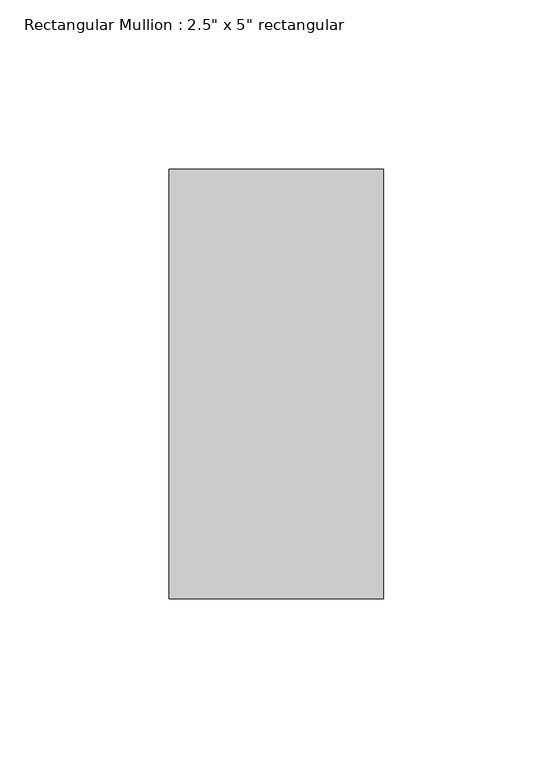
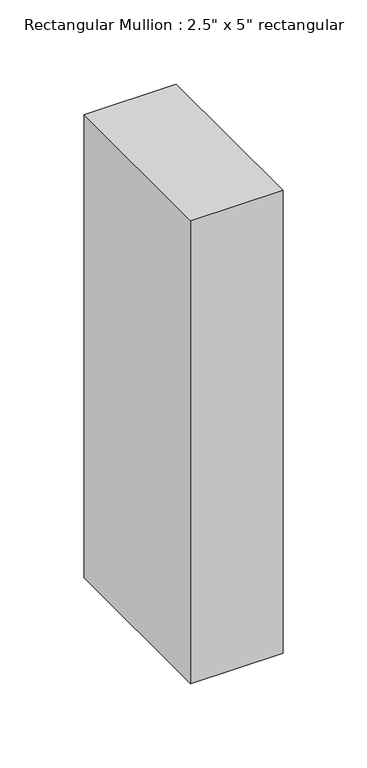
"""IFC4 building model written with IfcOpenShell, lengths in millimetres: member geometry."""

from ifc_helpers import new_model, si_unit, frame, origin, place, context, project, spatial, polyline, outline, extrude, source, transform, mapped, element, save


def member_02b8d6b6(model_context):
    return source(origin(), model_context, "Body", "SweptSolid", [
        extrude(outline(polyline([(0.0, 63.5), (0.0, -63.5), (-63.5, -63.5), (-63.5, 63.5), (0.0, 63.5)])), frame((0.0, 0.0, -336.55), z_axis=(0.0, 0.0, 1.0), x_axis=(1.0, 0.0, 0.0)), (0.0, 0.0, 1.0), 336.55),
    ])


if __name__ == "__main__":
    model = new_model("IFC4")
    model_context = context("Model", 3, world=origin())
    ifc_project = project(units=[si_unit("LENGTHUNIT", "METRE", prefix="MILLI")], contexts=[model_context])
    site = spatial("IfcSite", under=ifc_project)
    building = spatial("IfcBuilding", under=site)
    placement = place(None, origin())
    member_shape = member_02b8d6b6(model_context)
    element("IfcMember", 1, ObjectType="Rectangular Mullion : 2.5\" x 5\" rectangular", at=placement, inside=building, context=model_context, shape_type="MappedRepresentation", body=[
        mapped(member_shape, transform((0.0, 0.0, 0.0), x_axis=(1.0, 0.0, 0.0), y_axis=(0.0, 1.0, 0.0), z_axis=(0.0, 0.0, 1.0))),
    ])
    save(model, "model.ifc")

# Revit data of these elements
# Type "Rectangular Mullion : 2.5\" x 5\" rectangular"
#   built-in parameter 1007304 = 0.416667 (stored number, unit not read)
#   built-in parameter 1007301 = 0.104167 (stored number, unit not read)
#   built-in parameter 1007300 = 0.104167 (stored number, unit not read)
# Element 1 (IfcMember, "Rectangular Mullion : 2.5\" x 5\" rectangular")
#   Materials on its faces: "Aluminum"
# Materials
#   "Aluminum": class "Metal", colour RGB 247 247 247, transparency 0, Description = "Aluminum 6061", Cost = 0
